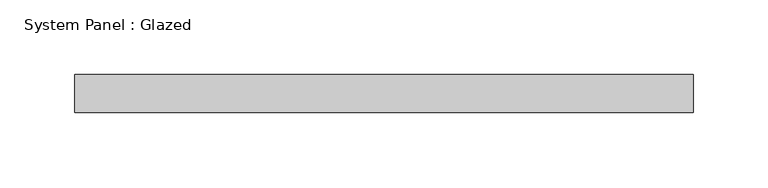
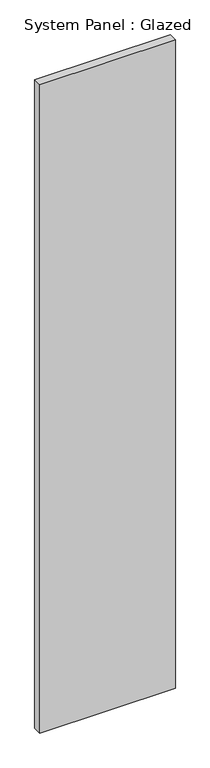
"""IFC4 building model written with IfcOpenShell, lengths in millimetres: plate geometry, System Panel : Glazed."""

from ifc_helpers import new_model, si_unit, origin, origin_with_axes, place, context, project, spatial, polyline, outline, extrude, source, transform, mapped, element, save


def system_panel_glazed_8c9d9dbc(model_context):
    return source(origin(), model_context, "Body", "SweptSolid", [
        extrude(outline(polyline([(206.375, -44.45), (-206.375, -44.45), (-206.375, -19.05), (206.375, -19.05), (206.375, -44.45)])), origin_with_axes(), (0.0, 0.0, 1.0), 2082.8),
    ])


if __name__ == "__main__":
    model = new_model("IFC4")
    model_context = context("Model", 3, world=origin())
    ifc_project = project(units=[si_unit("LENGTHUNIT", "METRE", prefix="MILLI")], contexts=[model_context])
    site = spatial("IfcSite", under=ifc_project)
    building = spatial("IfcBuilding", under=site)
    placement = place(None, origin())
    system_panel_glazed_shape = system_panel_glazed_8c9d9dbc(model_context)
    element("IfcPlate", 1, ObjectType="System Panel : Glazed", at=placement, inside=building, context=model_context, shape_type="MappedRepresentation", body=[
        mapped(system_panel_glazed_shape, transform((0.0, 0.0, 0.0), x_axis=(1.0, 0.0, 0.0), y_axis=(0.0, 1.0, 0.0), z_axis=(0.0, 0.0, 1.0))),
    ])
    save(model, "model.ifc")

# Revit data of these elements
# Type "System Panel : Glazed"
#   Construction Type Id = "GSP4R"
#   Analytic Construction = "1/8 in Pilkington single glazing"
#   Visual Light Transmittance = 0.9
#   Solar Heat Gain Coefficient = 0.86
#   Heat Transfer Coefficient (U) = 1.18115 BTU/(h·ft²·°F)
#   Define Thermal Properties by = 1
# Element 1 (IfcPlate, "System Panel : Glazed")
#   Materials on its faces: "Glass"
# Materials
#   "Glass": class "Glass", colour RGB 0 128 192, transparency 0.75, Description = "Soda Lime Glass", Cost = 0
